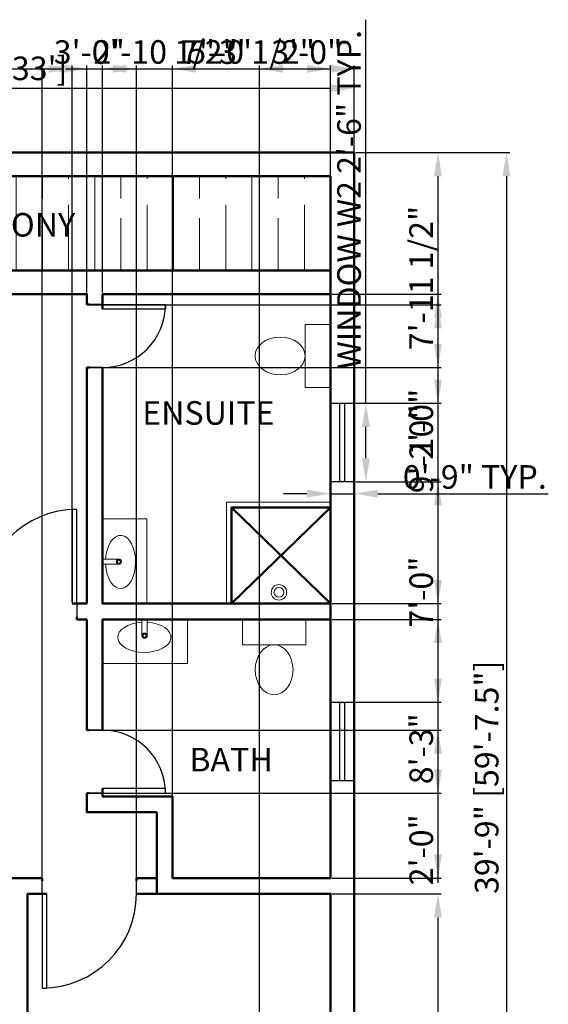
# Model space of a CAD drawing. Units: inches. Extents: x 2429 to 3343, y 1496 to 2530.
# Tile 7 of 7: x 3141 to 3343, y 2154 to 2530. Entities that reach past the tile are written whole.
import ezdxf

# ---------------------------------------------------------------- set-up
doc = ezdxf.new("R2010")
doc.units = ezdxf.units.IN
for name, color, linetype, lineweight in [('A-ANNO-DIMS', 2, 'Continuous', 18), ('A-AREA-IDEN', 3, 'Continuous', 18), ('A-DOOR', 3, 'Continuous', 25), ('A-FLOR-FIXT', 8, 'Continuous', 18), ('A-FLOR-PATT', 8, 'Continuous', 13), ('A-GLAZ', 4, 'Continuous', 25), ('A-WALL', 7, 'Continuous', 50)]:
    doc.layers.add(name, color=color, linetype=linetype, lineweight=lineweight)
doc.styles.get("Standard").update_dxf_attribs({"font": 'arial.ttf'})
doc.dimstyles.new('ISO-25', dxfattribs={"dimtxt": 9, "dimasz": 9, "dimexe": 1.25, "dimexo": 0.625, "dimtad": 1, "dimdec": 1, "dimlunit": 3, "dimtxsty": 'Standard', "dimcen": 9, "dimadec": 0, "dimazin": 0, "dimtfac": 1, "dimtdec": 1, "dimtmove": 0, "dimatfit": 3, "dimfxl": 1, "dimarcsym": 0})

# ---------------------------------------------------------------- blocks, each defined once
blk = doc.blocks.new('*D9')
at = {"layer": 'A-ANNO-DIMS', "color": 0, "lineweight": -2, "transparency": 16777216}
for p, q in [((3005.05, 2479.42), (3005.05, 2504.67)), ((3269.05, 2479.42), (3269.05, 2504.67)), ((3014.05, 2503.42), (3260.05, 2503.42))]:
    blk.add_line(p, q, dxfattribs=at)
at = {"layer": 'A-ANNO-DIMS', "color": 0, "transparency": 16777216}
for points in [[(3014.05, 2504.92), (3014.05, 2501.92), (3005.05, 2503.42)], [(3260.05, 2504.92), (3260.05, 2501.92), (3269.05, 2503.42)]]:
    blk.add_solid(points, dxfattribs=at)
at = {"layer": 'Defpoints', "color": 0, "transparency": 16777216}
for p in [(3269.05, 2503.42), (3005.05, 2478.79), (3269.05, 2478.79)]:
    blk.add_point(p, dxfattribs=at)
at = {"layer": 'A-ANNO-DIMS', "color": 0, "transparency": 16777216, "insert": (3137.05, 2509.81), "char_height": 9, "attachment_point": 5}
blk.add_mtext("22' [33']", dxfattribs=at)
blk = doc.blocks.new('*D10')
at = {"layer": 'A-ANNO-DIMS', "color": 0, "lineweight": -2, "transparency": 16777216}
for p, q in [((3270.09, 2478.79), (3328.44, 2478.79)), ((3327.19, 2469.79), (3327.19, 2010.79)), ((3269.67, 2001.79), (3328.44, 2001.79))]:
    blk.add_line(p, q, dxfattribs=at)
at = {"layer": 'A-ANNO-DIMS', "color": 0, "transparency": 16777216}
for points in [[(3325.69, 2469.79), (3328.69, 2469.79), (3327.19, 2478.79)], [(3325.69, 2010.79), (3328.69, 2010.79), (3327.19, 2001.79)]]:
    blk.add_solid(points, dxfattribs=at)
at = {"layer": 'Defpoints', "color": 0, "transparency": 16777216}
for p in [(3269.47, 2478.79), (3269.05, 2001.79), (3327.19, 2001.79)]:
    blk.add_point(p, dxfattribs=at)
at = {"layer": 'A-ANNO-DIMS', "color": 0, "transparency": 16777216, "insert": (3320.8, 2240.29), "char_height": 9, "attachment_point": 5, "rotation": 90}
blk.add_mtext('39\'-9" [59\'-7.5"]', dxfattribs=at)
blk = doc.blocks.new('*U2')
for p, q in [((0, 0), (0, -5)), ((-36, 0), (-36, -5))]:
    blk.add_line(p, q)
blk.add_lwpolyline([(0, 0), (0, 36), (-1.75, 36), (-1.75, 0)], close=True)
blk.add_arc((0, 0), 36, 90, 180)
blk = doc.blocks.new('*U4')
for p, q in [((0, 0), (0, 5)), ((24, 0), (24, 5))]:
    blk.add_line(p, q)
blk.add_lwpolyline([(0, 0), (0, -24), (1.75, -24), (1.75, 0)], close=True)
blk.add_arc((0, 0), 24, 270, 0)
blk = doc.blocks.new('*U11')
for p, q in [((-24, 0), (-24, 5)), ((0, 0), (0, 5))]:
    blk.add_line(p, q)
blk.add_lwpolyline([(0, 0), (0, -24), (-1.75, -24), (-1.75, 0)], close=True)
blk.add_arc((0, 0), 24, 180, 270)
blk = doc.blocks.new('*U13')
for p, q in [((0, 0), (0, 5)), ((36, 0), (36, 5))]:
    blk.add_line(p, q)
blk.add_lwpolyline([(0, 0), (0, -36), (1.75, -36), (1.75, 0)], close=True)
blk.add_arc((0, 0), 36, 270, 0)
blk = doc.blocks.new('WIN-PLAN-750')
for p, q in [((3.5, 0), (3.5, 30)), ((5.5, 0), (5.5, 30))]:
    blk.add_line(p, q)
blk.add_lwpolyline([(9, 30), (9, 0), (0, 0), (0, 30)], close=True)
blk = doc.blocks.new('*D27')
at = {"layer": 'A-ANNO-DIMS', "color": 0, "lineweight": -2, "transparency": 16777216}
for p, q in [((3273.55, 2383.07), (3273.55, 2529.56)), ((3269.67, 2383.07), (3274.8, 2383.07)), ((3273.55, 2362.07), (3273.55, 2374.07)), ((3269.67, 2353.07), (3274.8, 2353.07))]:
    blk.add_line(p, q, dxfattribs=at)
at = {"layer": 'A-ANNO-DIMS', "color": 0, "transparency": 16777216}
for points in [[(3272.05, 2374.07), (3275.05, 2374.07), (3273.55, 2383.07)], [(3272.05, 2362.07), (3275.05, 2362.07), (3273.55, 2353.07)]]:
    blk.add_solid(points, dxfattribs=at)
at = {"layer": 'Defpoints', "color": 0, "transparency": 16777216}
for p in [(3269.05, 2383.07), (3273.55, 2383.07), (3269.05, 2353.07)]:
    blk.add_point(p, dxfattribs=at)
at = {"layer": 'A-ANNO-DIMS', "color": 0, "transparency": 16777216, "insert": (3268.27, 2460.81), "char_height": 9, "attachment_point": 5, "rotation": 90}
blk.add_mtext('WINDOW W2 2\'-6" TYP.', dxfattribs=at)
blk = doc.blocks.new('*D28')
at = {"layer": 'A-ANNO-DIMS', "color": 0, "lineweight": -2, "transparency": 16777216}
for p, q in [((3260.05, 2352.44), (3260.05, 2347.32)), ((3269.05, 2352.44), (3269.05, 2347.32)), ((3251.05, 2348.57), (3242.05, 2348.57)), ((3260.05, 2348.57), (3269.05, 2348.57)), ((3278.05, 2348.57), (3343.16, 2348.57))]:
    blk.add_line(p, q, dxfattribs=at)
at = {"layer": 'A-ANNO-DIMS', "color": 0, "transparency": 16777216}
for points in [[(3251.05, 2350.07), (3251.05, 2347.07), (3260.05, 2348.57)], [(3278.05, 2350.07), (3278.05, 2347.07), (3269.05, 2348.57)]]:
    blk.add_solid(points, dxfattribs=at)
at = {"layer": 'Defpoints', "color": 0, "transparency": 16777216}
for p in [(3260.05, 2353.07), (3269.05, 2353.07), (3269.05, 2348.57)]:
    blk.add_point(p, dxfattribs=at)
at = {"layer": 'A-ANNO-DIMS', "color": 0, "transparency": 16777216, "insert": (3315.1, 2353.79), "char_height": 9, "attachment_point": 5}
blk.add_mtext('0\'-9" TYP.', dxfattribs=at)
blk = doc.blocks.new('*D58')
at = {"layer": 'A-ANNO-DIMS', "color": 0, "lineweight": -2, "transparency": 16777216}
for p, q in [((3014.05, 2425.42), (3014.05, 2512.04)), ((3167.05, 2425.42), (3167.05, 2512.04)), ((3023.05, 2510.79), (3158.05, 2510.79))]:
    blk.add_line(p, q, dxfattribs=at)
at = {"layer": 'A-ANNO-DIMS', "color": 0, "transparency": 16777216}
for points in [[(3023.05, 2512.29), (3023.05, 2509.29), (3014.05, 2510.79)], [(3158.05, 2512.29), (3158.05, 2509.29), (3167.05, 2510.79)]]:
    blk.add_solid(points, dxfattribs=at)
at = {"layer": 'Defpoints', "color": 0, "transparency": 16777216}
for p in [(3167.05, 2510.79), (3014.05, 2424.79), (3167.05, 2424.79)]:
    blk.add_point(p, dxfattribs=at)
at = {"layer": 'A-ANNO-DIMS', "color": 0, "transparency": 16777216, "insert": (3090.55, 2516.01), "char_height": 9, "attachment_point": 5}
blk.add_mtext('12\'-9"', dxfattribs=at)
blk = doc.blocks.new('*D60')
at = {"layer": 'A-ANNO-DIMS', "color": 0, "lineweight": -2, "transparency": 16777216}
for p, q in [((3173.05, 2425.42), (3173.05, 2512.04)), ((3260.05, 2425.42), (3260.05, 2512.04)), ((3182.05, 2510.79), (3251.05, 2510.79))]:
    blk.add_line(p, q, dxfattribs=at)
at = {"layer": 'A-ANNO-DIMS', "color": 0, "transparency": 16777216}
for points in [[(3182.05, 2512.29), (3182.05, 2509.29), (3173.05, 2510.79)], [(3251.05, 2512.29), (3251.05, 2509.29), (3260.05, 2510.79)]]:
    blk.add_solid(points, dxfattribs=at)
at = {"layer": 'Defpoints', "color": 0, "transparency": 16777216}
for p in [(3260.05, 2510.79), (3173.05, 2424.79), (3260.05, 2424.79)]:
    blk.add_point(p, dxfattribs=at)
at = {"layer": 'A-ANNO-DIMS', "color": 0, "transparency": 16777216, "insert": (3216.55, 2516.02), "char_height": 9, "attachment_point": 5}
blk.add_mtext('7\'-3"', dxfattribs=at)
blk = doc.blocks.new('*D61')
at = {"layer": 'A-ANNO-DIMS', "color": 0, "lineweight": -2, "transparency": 16777216}
for p, q in [((3260.67, 2424.79), (3302.3, 2424.79)), ((3301.05, 2415.79), (3301.05, 2315.58)), ((3260.67, 2306.58), (3302.3, 2306.58))]:
    blk.add_line(p, q, dxfattribs=at)
at = {"layer": 'A-ANNO-DIMS', "color": 0, "transparency": 16777216}
for points in [[(3299.55, 2415.79), (3302.55, 2415.79), (3301.05, 2424.79)], [(3299.55, 2315.58), (3302.55, 2315.58), (3301.05, 2306.58)]]:
    blk.add_solid(points, dxfattribs=at)
at = {"layer": 'Defpoints', "color": 0, "transparency": 16777216}
for p in [(3260.05, 2424.79), (3260.05, 2306.58), (3301.05, 2306.58)]:
    blk.add_point(p, dxfattribs=at)
at = {"layer": 'A-ANNO-DIMS', "color": 0, "transparency": 16777216, "insert": (3295.83, 2365.69), "char_height": 9, "attachment_point": 5, "rotation": 90}
blk.add_mtext('9\'-10"', dxfattribs=at)
blk = doc.blocks.new('*D62')
at = {"layer": 'A-ANNO-DIMS', "color": 0, "lineweight": -2, "transparency": 16777216}
for p, q in [((3260.67, 2300.58), (3302.3, 2300.58)), ((3301.05, 2291.58), (3301.05, 2210.79)), ((3260.67, 2201.79), (3302.3, 2201.79))]:
    blk.add_line(p, q, dxfattribs=at)
at = {"layer": 'A-ANNO-DIMS', "color": 0, "transparency": 16777216}
for points in [[(3299.55, 2291.58), (3302.55, 2291.58), (3301.05, 2300.58)], [(3299.55, 2210.79), (3302.55, 2210.79), (3301.05, 2201.79)]]:
    blk.add_solid(points, dxfattribs=at)
at = {"layer": 'Defpoints', "color": 0, "transparency": 16777216}
for p in [(3260.05, 2300.58), (3260.05, 2201.79), (3301.05, 2201.79)]:
    blk.add_point(p, dxfattribs=at)
at = {"layer": 'A-ANNO-DIMS', "color": 0, "transparency": 16777216, "insert": (3295.83, 2251.18), "char_height": 9, "attachment_point": 5, "rotation": 90}
blk.add_mtext('8\'-3"', dxfattribs=at)
blk = doc.blocks.new('*D68')
at = {"layer": 'A-ANNO-DIMS', "color": 0, "lineweight": -2, "transparency": 16777216}
for p, q in [((3260.67, 2195.79), (3302.3, 2195.79)), ((3301.05, 2186.79), (3301.05, 2036.79)), ((3260.67, 2027.79), (3302.3, 2027.79))]:
    blk.add_line(p, q, dxfattribs=at)
at = {"layer": 'A-ANNO-DIMS', "color": 0, "transparency": 16777216}
for points in [[(3299.55, 2186.79), (3302.55, 2186.79), (3301.05, 2195.79)], [(3299.55, 2036.79), (3302.55, 2036.79), (3301.05, 2027.79)]]:
    blk.add_solid(points, dxfattribs=at)
at = {"layer": 'Defpoints', "color": 0, "transparency": 16777216}
for p in [(3260.05, 2195.79), (3260.05, 2027.79), (3301.05, 2027.79)]:
    blk.add_point(p, dxfattribs=at)
at = {"layer": 'A-ANNO-DIMS', "color": 0, "transparency": 16777216, "insert": (3295.83, 2111.79), "char_height": 9, "attachment_point": 5, "rotation": 90}
blk.add_mtext('14\'-0"', dxfattribs=at)
blk = doc.blocks.new('*D74')
at = {"layer": 'A-ANNO-DIMS', "color": 0, "lineweight": -2, "transparency": 16777216}
for p, q in [((3269.67, 2478.79), (3302.3, 2478.79)), ((3301.05, 2469.79), (3301.05, 2392.07)), ((3269.67, 2383.07), (3302.3, 2383.07))]:
    blk.add_line(p, q, dxfattribs=at)
at = {"layer": 'A-ANNO-DIMS', "color": 0, "transparency": 16777216}
for points in [[(3299.55, 2469.79), (3302.55, 2469.79), (3301.05, 2478.79)], [(3299.55, 2392.07), (3302.55, 2392.07), (3301.05, 2383.07)]]:
    blk.add_solid(points, dxfattribs=at)
at = {"layer": 'Defpoints', "color": 0, "transparency": 16777216}
for p in [(3269.05, 2478.79), (3269.05, 2383.07), (3301.05, 2383.07)]:
    blk.add_point(p, dxfattribs=at)
at = {"layer": 'A-ANNO-DIMS', "color": 0, "transparency": 16777216, "insert": (3295.77, 2430.93), "char_height": 9, "attachment_point": 5, "rotation": 90}
blk.add_mtext('7\'-11 1/2"', dxfattribs=at)
blk = doc.blocks.new('*D75')
at = {"layer": 'A-ANNO-DIMS', "color": 0, "lineweight": -2, "transparency": 16777216}
for p, q in [((3269.67, 2353.07), (3302.3, 2353.07)), ((3301.05, 2344.07), (3301.05, 2277.95)), ((3269.67, 2268.95), (3302.3, 2268.95))]:
    blk.add_line(p, q, dxfattribs=at)
at = {"layer": 'A-ANNO-DIMS', "color": 0, "transparency": 16777216}
for points in [[(3299.55, 2344.07), (3302.55, 2344.07), (3301.05, 2353.07)], [(3299.55, 2277.95), (3302.55, 2277.95), (3301.05, 2268.95)]]:
    blk.add_solid(points, dxfattribs=at)
at = {"layer": 'Defpoints', "color": 0, "transparency": 16777216}
for p in [(3269.05, 2353.07), (3269.05, 2268.95), (3301.05, 2268.95)]:
    blk.add_point(p, dxfattribs=at)
at = {"layer": 'A-ANNO-DIMS', "color": 0, "transparency": 16777216, "insert": (3295.83, 2311.01), "char_height": 9, "attachment_point": 5, "rotation": 90}
blk.add_mtext('7\'-0"', dxfattribs=at)
blk = doc.blocks.new('*D77')
at = {"layer": 'A-ANNO-DIMS', "color": 0, "lineweight": -2, "transparency": 16777216}
for p, q in [((3232.91, 2019.41), (3232.91, 2512.04)), ((3269.05, 2019.41), (3269.05, 2512.04)), ((3241.91, 2510.79), (3260.05, 2510.79))]:
    blk.add_line(p, q, dxfattribs=at)
at = {"layer": 'A-ANNO-DIMS', "color": 0, "transparency": 16777216}
for points in [[(3241.91, 2512.29), (3241.91, 2509.29), (3232.91, 2510.79)], [(3260.05, 2512.29), (3260.05, 2509.29), (3269.05, 2510.79)]]:
    blk.add_solid(points, dxfattribs=at)
at = {"layer": 'Defpoints', "color": 0, "transparency": 16777216}
for p in [(3269.05, 2510.79), (3232.91, 2018.79), (3269.05, 2018.79)]:
    blk.add_point(p, dxfattribs=at)
at = {"layer": 'A-ANNO-DIMS', "color": 0, "transparency": 16777216, "insert": (3250.98, 2516.02), "char_height": 9, "attachment_point": 5}
blk.add_mtext('3\'-0"', dxfattribs=at)
blk = doc.blocks.new('*D78')
at = {"layer": 'A-ANNO-DIMS', "color": 0, "lineweight": -2, "transparency": 16777216}
for p, q in [((3167.67, 2420.74), (3302.3, 2420.74)), ((3301.05, 2411.74), (3301.05, 2405.74)), ((3167.67, 2396.74), (3302.3, 2396.74)), ((3301.05, 2396.74), (3301.05, 2362.41))]:
    blk.add_line(p, q, dxfattribs=at)
at = {"layer": 'A-ANNO-DIMS', "color": 0, "transparency": 16777216}
for points in [[(3299.55, 2411.74), (3302.55, 2411.74), (3301.05, 2420.74)], [(3299.55, 2405.74), (3302.55, 2405.74), (3301.05, 2396.74)]]:
    blk.add_solid(points, dxfattribs=at)
at = {"layer": 'Defpoints', "color": 0, "transparency": 16777216}
for p in [(3167.05, 2420.74), (3167.05, 2396.74), (3301.05, 2396.74)]:
    blk.add_point(p, dxfattribs=at)
at = {"layer": 'A-ANNO-DIMS', "color": 0, "transparency": 16777216, "insert": (3295.83, 2375.08), "char_height": 9, "attachment_point": 5, "rotation": 90}
blk.add_mtext('2\'-0"', dxfattribs=at)
blk = doc.blocks.new('*D79')
at = {"layer": 'A-ANNO-DIMS', "color": 0, "lineweight": -2, "transparency": 16777216}
for p, q in [((3127.2, 2307.21), (3127.2, 2512.04)), ((3161.45, 2307.21), (3161.45, 2512.04)), ((3136.2, 2510.79), (3152.45, 2510.79)), ((3161.45, 2510.79), (3223.74, 2510.79))]:
    blk.add_line(p, q, dxfattribs=at)
at = {"layer": 'A-ANNO-DIMS', "color": 0, "transparency": 16777216}
for points in [[(3136.2, 2512.29), (3136.2, 2509.29), (3127.2, 2510.79)], [(3152.45, 2512.29), (3152.45, 2509.29), (3161.45, 2510.79)]]:
    blk.add_solid(points, dxfattribs=at)
at = {"layer": 'Defpoints', "color": 0, "transparency": 16777216}
for p in [(3161.45, 2510.79), (3127.2, 2306.58), (3161.45, 2306.58)]:
    blk.add_point(p, dxfattribs=at)
at = {"layer": 'A-ANNO-DIMS', "color": 0, "transparency": 16777216, "insert": (3197.09, 2516.07), "char_height": 9, "attachment_point": 5}
blk.add_mtext('2\'-10 1/2"', dxfattribs=at)
blk = doc.blocks.new('*D80')
at = {"layer": 'A-ANNO-DIMS', "color": 0, "lineweight": -2, "transparency": 16777216}
for p, q in [((3167.67, 2258.27), (3302.3, 2258.27)), ((3301.05, 2249.27), (3301.05, 2243.27)), ((3167.67, 2234.27), (3302.3, 2234.27)), ((3301.05, 2234.27), (3301.05, 2199.94))]:
    blk.add_line(p, q, dxfattribs=at)
at = {"layer": 'A-ANNO-DIMS', "color": 0, "transparency": 16777216}
for points in [[(3299.55, 2249.27), (3302.55, 2249.27), (3301.05, 2258.27)], [(3299.55, 2243.27), (3302.55, 2243.27), (3301.05, 2234.27)]]:
    blk.add_solid(points, dxfattribs=at)
at = {"layer": 'Defpoints', "color": 0, "transparency": 16777216}
for p in [(3167.05, 2258.27), (3167.05, 2234.27), (3301.05, 2234.27)]:
    blk.add_point(p, dxfattribs=at)
at = {"layer": 'A-ANNO-DIMS', "color": 0, "transparency": 16777216, "insert": (3295.83, 2212.61), "char_height": 9, "attachment_point": 5, "rotation": 90}
blk.add_mtext('2\'-0"', dxfattribs=at)
blk = doc.blocks.new('*D82')
at = {"layer": 'A-ANNO-DIMS', "color": 0, "lineweight": -2, "transparency": 16777216}
for p, q in [((3149.97, 2196.41), (3149.97, 2512.04)), ((3185.97, 2196.41), (3185.97, 2512.04)), ((3158.97, 2510.79), (3176.97, 2510.79))]:
    blk.add_line(p, q, dxfattribs=at)
at = {"layer": 'A-ANNO-DIMS', "color": 0, "transparency": 16777216}
for points in [[(3158.97, 2512.29), (3158.97, 2509.29), (3149.97, 2510.79)], [(3176.97, 2512.29), (3176.97, 2509.29), (3185.97, 2510.79)]]:
    blk.add_solid(points, dxfattribs=at)
at = {"layer": 'Defpoints', "color": 0, "transparency": 16777216}
for p in [(3185.97, 2510.79), (3149.97, 2195.79), (3185.97, 2195.79)]:
    blk.add_point(p, dxfattribs=at)
at = {"layer": 'A-ANNO-DIMS', "color": 0, "transparency": 16777216, "insert": (3167.97, 2516.02), "char_height": 9, "attachment_point": 5}
blk.add_mtext('3\'-0"', dxfattribs=at)
blk = doc.blocks.new('*D83')
at = {"layer": 'A-ANNO-DIMS', "color": 0, "lineweight": -2, "transparency": 16777216}
for p, q in [((3199.75, 2202.41), (3199.75, 2512.04)), ((3260.05, 2202.41), (3260.05, 2512.04)), ((3208.75, 2510.79), (3251.05, 2510.79))]:
    blk.add_line(p, q, dxfattribs=at)
at = {"layer": 'A-ANNO-DIMS', "color": 0, "transparency": 16777216}
for points in [[(3208.75, 2512.29), (3208.75, 2509.29), (3199.75, 2510.79)], [(3251.05, 2512.29), (3251.05, 2509.29), (3260.05, 2510.79)]]:
    blk.add_solid(points, dxfattribs=at)
at = {"layer": 'Defpoints', "color": 0, "transparency": 16777216}
for p in [(3260.05, 2510.79), (3199.75, 2201.79), (3260.05, 2201.79)]:
    blk.add_point(p, dxfattribs=at)
at = {"layer": 'A-ANNO-DIMS', "color": 0, "transparency": 16777216, "insert": (3229.9, 2516.07), "char_height": 9, "attachment_point": 5}
blk.add_mtext('5\'-0 1/2"', dxfattribs=at)

msp = doc.modelspace()

# ---------------------------------------------------------------- hatches: boundary and pattern name
at = {"layer": 'A-FLOR-FIXT'}
h = msp.add_hatch(color=256, dxfattribs=at)
h.dxf.hatch_style = 1
h.paths.add_polyline_path([(3179.27593, 2321.61819, 1), (3179.27593, 2323.61819, 1)])
h.paths.add_polyline_path([(3179.27593, 2323.18065, -1), (3179.27593, 2322.05572, -1)], flags=16)
h = msp.add_hatch(color=256, dxfattribs=at)
h.dxf.hatch_style = 1
h.paths.add_polyline_path([(3188.08405, 2294.355, 1), (3190.08405, 2294.355, 1)])
h.paths.add_polyline_path([(3189.64652, 2294.355, -1), (3188.52159, 2294.355, -1)], flags=16)
at = {"layer": 'A-FLOR-PATT'}
h = msp.add_hatch(dxfattribs=at)
h.set_pattern_fill('GOST_WOOD', color=256, scale=5)
h.set_pattern_definition([(90, (3260.048, 2433.792), (30, -2e-15), [50, -10]), (90, (3270.048, 2423.792), (30, -2e-15), [30, -7.5, 15, -7.5]), (90, (3280.048, 2408.792), (30, -2e-15), [50, -10])])
h.paths.add_polyline_path([(3260.04839, 2469.7918), (3014.04839, 2469.7918), (3014.04839, 2433.7918), (3260.04839, 2433.7918)])
h.paths.add_polyline_path([(3104.56895, 2440.5916), (3163.9551, 2440.5916), (3163.9551, 2462.39929), (3104.56895, 2462.39929)], flags=24)

# ---------------------------------------------------------------- linework, layer by layer
at = {"layer": 'A-FLOR-FIXT'}
for points in [[(3260.04839, 2389.11593), (3260.04839, 2413.22093), (3250.32664, 2413.22093), (3250.32664, 2389.11593)], [(3173.04839, 2339.0198), (3173.04839, 2306.58253), (3189.96468, 2306.58253), (3189.96468, 2339.0198)], [(3205.48566, 2300.58253), (3173.04839, 2300.58253), (3173.04839, 2283.66624), (3205.48566, 2283.66624)], [(3250.56997, 2300.58253), (3226.46497, 2300.58253), (3226.46497, 2290.86078), (3250.56997, 2290.86078)]]:
    msp.add_lwpolyline(points, close=True, dxfattribs=at)
msp.add_lwpolyline([(3220.29148, 2306.58253), (3220.29148, 2345.34148), (3260.04839, 2345.34148)], dxfattribs=at)
for points in [[(3173.04839, 2321.61819), (3179.27593, 2321.61819, 1), (3179.27593, 2323.61819), (3173.04839, 2323.61819)], [(3188.08405, 2300.58253), (3188.08405, 2294.355, 1), (3190.08405, 2294.355), (3190.08405, 2300.58253)]]:
    msp.add_lwpolyline(points, format="xyb", dxfattribs=at)
for centre, radius in [((3179.21346, 2322.61624), 1), ((3179.27593, 2322.61819), 0.56247), ((3240.36016, 2310.89557), 2.95892), ((3240.36016, 2310.89557), 2.95892), ((3240.36016, 2310.89557), 2.95892), ((3240.36016, 2310.89557), 1.90092), ((3189.0821, 2294.41746), 1), ((3189.08405, 2294.355), 0.56247)]:
    msp.add_circle(centre, radius, dxfattribs=at)
for centre, major_axis in [((3240.79957, 2401.16843), (-9.52707, 0)), ((3238.51747, 2281.33371), (0, -9.52707))]:
    msp.add_ellipse(centre, major_axis=major_axis, ratio=0.757824975, dxfattribs=at)
for centre, major_axis in [((3179.90899, 2322.50886), (0, 10.16289)), ((3188.97472, 2293.72193), (10.16289, 0))]:
    msp.add_ellipse(centre, major_axis=major_axis, ratio=0.564616754, start_param=1.65854801, end_param=7.744608334, dxfattribs=at)
at = {"layer": 'A-WALL'}
for p, q in [((3168.04839, 2420.74151), (3167.04839, 2420.74151)), ((3168.04839, 2396.74151), (3167.04839, 2396.74151)), ((3163.19704, 2301.58253), (3163.19704, 2300.58253)), ((3163.19704, 2300.58253), (3167.04839, 2300.58253)), ((3168.04839, 2258.27036), (3167.04839, 2258.27036)), ((3168.04839, 2234.27036), (3167.04839, 2234.27036)), ((3149.96707, 2200.78649), (3149.96707, 2201.78649)), ((3185.96707, 2200.78649), (3185.96707, 2201.78649))]:
    msp.add_line(p, q, dxfattribs=at)
for points in [[(3135.41055, 1970.47184), (3269.04839, 1970.47184), (3269.04839, 2001.78649), (3269.04839, 2325.78649), (3269.04839, 2478.7918), (3005.04839, 2478.7918), (3005.04839, 2325.78649), (3005.04839, 2319.78649), (3005.04839, 2199.78649), (3005.04839, 2018.78649), (3135.41055, 2018.78649)], [(3260.04839, 2469.7918), (3014.04839, 2469.7918), (3014.04839, 2433.7918), (3260.04839, 2433.7918)], [(3185.96707, 2201.78649), (3193.74506, 2201.78649)]]:
    msp.add_lwpolyline(points, close=True, dxfattribs=at)
for points in [[(3260.04839, 2236.50016), (3260.04839, 2325.78649), (3260.04839, 2469.7918)], [(3127.19704, 2306.58253), (3014.04839, 2306.58253), (3014.04839, 2319.78649), (3014.04839, 2325.78649), (3014.04839, 2424.7918), (3167.04839, 2424.7918), (3167.04839, 2420.74151)], [(3260.04839, 2373.7918), (3260.04839, 2424.7918), (3173.04839, 2424.7918), (3173.04839, 2418.99151)], [(3167.04839, 2396.74151), (3167.04839, 2306.58253)], [(3173.04839, 2396.74151), (3173.04839, 2306.58253), (3260.04839, 2306.58253), (3222.29148, 2343.34148), (3260.04839, 2343.34148), (3222.29148, 2306.58253), (3222.29148, 2343.34148)], [(3167.04839, 2306.58253), (3161.44704, 2306.58253)], [(3167.04839, 2300.58253), (3167.04839, 2258.27036)], [(3173.04839, 2258.27036), (3173.04839, 2300.58253), (3260.04839, 2300.58253)], [(3260.04839, 2249.7918), (3260.04839, 2201.78649), (3199.74506, 2201.78649), (3199.74506, 2232.92773), (3173.04839, 2232.92773), (3173.04839, 2236.02036)], [(3167.04839, 2234.27036), (3167.04839, 2226.92773), (3193.74506, 2226.92773), (3193.74506, 2201.78649), (3193.74506, 2195.78649)], [(3149.96707, 2201.78649), (3135.7165, 2201.78649)], [(3185.96707, 2195.78649), (3260.04839, 2195.78649), (3260.04839, 2027.78649), (3144.41055, 2027.78649), (3144.41055, 2195.78649), (3151.71707, 2195.78649)]]:
    msp.add_lwpolyline(points, dxfattribs=at)

# ---------------------------------------------------------------- block references
at = {"layer": 'A-DOOR', "rotation": 90}
for name, p in [('*U11', (3173.04839, 2420.74151)), ('*U4', (3173.04839, 2234.27036))]:
    msp.add_blockref(name, p, dxfattribs=at)
at = {"layer": 'A-DOOR'}
for name, p in [('*U2', (3163.19704, 2306.58253)), ('*U13', (3149.96707, 2195.78649))]:
    msp.add_blockref(name, p, dxfattribs=at)
at = {"layer": 'A-GLAZ'}
for p in [(3260.04882, 2353.06575), (3260.04882, 2238.94871)]:
    msp.add_blockref('WIN-PLAN-750', p, dxfattribs=at)

# ---------------------------------------------------------------- texts
at = {"layer": 'A-AREA-IDEN', "char_height": 9, "attachment_point": 1}
for s, width, insert in [('{\\fCalibri|b0|i0|c0|p34;BALCONY}', 63.8011805, (3108.00972, 2455.73929)), ('{\\fCalibri|b0|i0|c0|p34;ENSUITE}', 51.2251285, (3188.19866, 2383.89199)), ('{\\fCalibri|b0|i0|c0|p34;BATH}', 51.2251285, (3206.16355, 2251.51441))]:
    msp.add_mtext_dynamic_manual_height_columns(s, width=width, gutter_width=12.5, heights=[0], dxfattribs=dict(at, insert=insert))

# ---------------------------------------------------------------- dimensions: what is measured, and where the dimension line sits
at = {"layer": 'A-ANNO-DIMS'}
for base, p1, p2, override, picture, middle in [((3161.447043, 2510.791805), (3127.197043, 2306.582531), (3161.447043, 2306.582531), {"dimdec": 1, "dimlfac": 1, "dimrnd": 0, "dimzin": 1, "dimdsep": 46, "dimlunit": 4, "dimfrac": 2}, '*D79', (3197.0928479113, 2516.070283854)), ((3260.04839, 2510.7918), (3199.74506, 2201.78649), (3260.04839, 2201.78649), {"dimdec": 1, "dimlfac": 1, "dimrnd": 0, "dimzin": 1, "dimdsep": 46, "dimlunit": 4, "dimfrac": 2}, '*D83', (3229.89673, 2516.07028)), ((3269.04839, 2503.41546), (3005.04839, 2478.7918), (3269.04839, 2478.7918), {"dimclrd": 0, "dimclre": 0, "dimclrt": 0}, '*D9', (3137.04839, 2509.8082)), ((3167.04839, 2510.7918), (3014.04839, 2424.7918), (3167.04839, 2424.7918), {"dimdec": 1, "dimlfac": 1, "dimrnd": 0, "dimzin": 1, "dimdsep": 46, "dimlunit": 4, "dimfrac": 2}, '*D58', (3090.54839, 2516.01196)), ((3185.96707, 2510.7918), (3149.96707, 2195.78649), (3185.96707, 2195.78649), {"dimdec": 1, "dimlfac": 1, "dimrnd": 0, "dimzin": 1, "dimdsep": 46, "dimlunit": 4, "dimfrac": 2}, '*D82', (3167.96707, 2516.01503)), ((3260.04839, 2510.7918), (3173.04839, 2424.7918), (3260.04839, 2424.7918), {"dimdec": 1, "dimlfac": 1, "dimrnd": 0, "dimzin": 1, "dimdsep": 46, "dimlunit": 4, "dimfrac": 2}, '*D60', (3216.54839, 2516.01503)), ((3269.04839, 2510.7918), (3232.90545, 2018.78649), (3269.04839, 2018.78649), {"dimdec": 1, "dimlfac": 1, "dimrnd": 0, "dimzin": 1, "dimdsep": 46, "dimlunit": 4, "dimfrac": 2}, '*D77', (3250.97692, 2516.01503))]:
    dim = msp.add_linear_dim(base=base, p1=p1, p2=p2, dimstyle='ISO-25', override=override, dxfattribs=at)
    dim.commit()
    dim.dimension.update_dxf_attribs({"geometry": picture, "text_midpoint": middle})
dim = msp.add_linear_dim(base=(3273.54839, 2383.06613), p1=(3269.04839, 2353.06613), p2=(3269.04839, 2383.06613), angle=90, text='WINDOW W2 <> TYP.', dimstyle='ISO-25', override={"dimdec": 1, "dimlfac": 1, "dimrnd": 0, "dimzin": 1, "dimdsep": 46, "dimlunit": 4, "dimfrac": 2}, dxfattribs=at)
dim.commit()
dim.dimension.update_dxf_attribs({"geometry": '*D27', "text_midpoint": (3268.26684, 2460.81118)})
for base, p1, p2, override, picture, middle in [((3301.04839, 2383.06613), (3269.04839, 2478.7918), (3269.04839, 2383.06613), {"dimdec": 1, "dimlfac": 1, "dimrnd": 0, "dimzin": 1, "dimdsep": 46, "dimlunit": 4, "dimfrac": 2}, '*D74', (3295.76991, 2430.92897)), ((3327.19291, 2001.78649), (3269.46607, 2478.7918), (3269.04839, 2001.78649), {"dimclrd": 0, "dimclre": 0, "dimclrt": 0}, '*D10', (3320.80018, 2240.28915)), ((3301.04839, 2306.58253), (3260.04839, 2424.7918), (3260.04839, 2306.58253), {"dimdec": 1, "dimlfac": 1, "dimrnd": 0, "dimzin": 1, "dimdsep": 46, "dimlunit": 4, "dimfrac": 2}, '*D61', (3295.82824, 2365.68717)), ((3301.04839, 2396.74151), (3167.04839, 2420.74151), (3167.04839, 2396.74151), {"dimdec": 1, "dimlfac": 1, "dimrnd": 0, "dimzin": 1, "dimdsep": 46, "dimlunit": 4, "dimfrac": 2}, '*D78', (3295.82824, 2375.07763)), ((3301.04839, 2268.94909), (3269.04839, 2353.06613), (3269.04839, 2268.94909), {"dimdec": 1, "dimlfac": 1, "dimrnd": 0, "dimzin": 1, "dimdsep": 46, "dimlunit": 4, "dimfrac": 2}, '*D75', (3295.82824, 2311.00761)), ((3301.04839, 2201.78649), (3260.04839, 2300.58253), (3260.04839, 2201.78649), {"dimdec": 1, "dimlfac": 1, "dimrnd": 0, "dimzin": 1, "dimdsep": 46, "dimlunit": 4, "dimfrac": 2}, '*D62', (3295.82517, 2251.18451)), ((3301.04839, 2234.27036), (3167.04839, 2258.27036), (3167.04839, 2234.27036), {"dimdec": 1, "dimlfac": 1, "dimrnd": 0, "dimzin": 1, "dimdsep": 46, "dimlunit": 4, "dimfrac": 2}, '*D80', (3295.82824, 2212.60647)), ((3301.04839, 2027.78649), (3260.04839, 2195.78649), (3260.04839, 2027.78649), {"dimdec": 1, "dimlfac": 1, "dimrnd": 0, "dimzin": 1, "dimdsep": 46, "dimlunit": 4, "dimfrac": 2}, '*D68', (3295.82824, 2111.78649))]:
    dim = msp.add_linear_dim(base=base, p1=p1, p2=p2, angle=90, dimstyle='ISO-25', override=override, dxfattribs=at)
    dim.commit()
    dim.dimension.update_dxf_attribs({"geometry": picture, "text_midpoint": middle})
dim = msp.add_linear_dim(base=(3269.04839, 2348.56613), p1=(3260.04839, 2353.06613), p2=(3269.04839, 2353.06613), text='<> TYP.', dimstyle='ISO-25', override={"dimdec": 1, "dimlfac": 1, "dimrnd": 0, "dimzin": 1, "dimdsep": 46, "dimlunit": 4, "dimfrac": 2}, dxfattribs=at)
dim.commit()
dim.dimension.update_dxf_attribs({"geometry": '*D28', "text_midpoint": (3315.10313, 2353.78628)})

doc.saveas('drawing.dxf')
